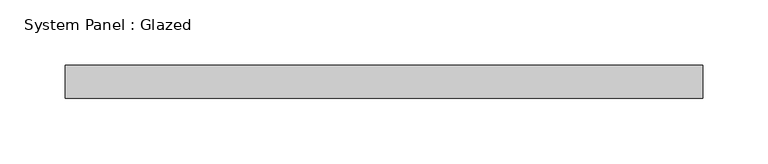
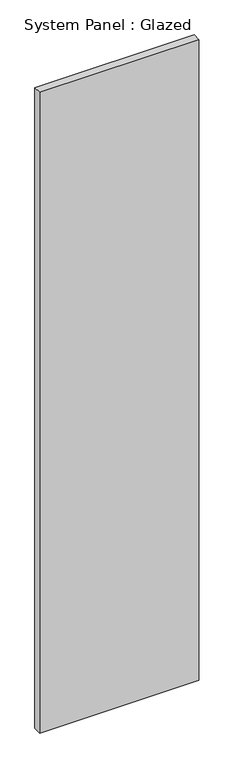
"""IFC4 building model written with IfcOpenShell, lengths in millimetres: plate geometry, System Panel : Glazed."""

from ifc_helpers import new_model, si_unit, origin, origin_with_axes, place, context, project, spatial, polyline, outline, extrude, source, transform, mapped, element, save


def system_panel_glazed_b4762422(model_context):
    return source(origin(), model_context, "Body", "SweptSolid", [
        extrude(outline(polyline([(244.9190503, -44.45), (-244.9190503, -44.45), (-244.9190503, -19.05), (244.9190503, -19.05), (244.9190503, -44.45)])), origin_with_axes(), (0.0, 0.0, 1.0), 2082.8),
    ])


if __name__ == "__main__":
    model = new_model("IFC4")
    model_context = context("Model", 3, world=origin())
    ifc_project = project(units=[si_unit("LENGTHUNIT", "METRE", prefix="MILLI")], contexts=[model_context])
    site = spatial("IfcSite", under=ifc_project)
    building = spatial("IfcBuilding", under=site)
    placement = place(None, origin())
    system_panel_glazed_shape = system_panel_glazed_b4762422(model_context)
    element("IfcPlate", 1, ObjectType="System Panel : Glazed", at=placement, inside=building, context=model_context, shape_type="MappedRepresentation", body=[
        mapped(system_panel_glazed_shape, transform((0.0, 0.0, 0.0), x_axis=(1.0, 0.0, 0.0), y_axis=(0.0, 1.0, 0.0), z_axis=(0.0, 0.0, 1.0))),
    ])
    save(model, "model.ifc")

# Revit data of these elements
# Type "System Panel : Glazed"
#   Construction Type Id = "GSP4R"
#   Analytic Construction = "1/8 in Pilkington single glazing"
#   Visual Light Transmittance = 0.9
#   Solar Heat Gain Coefficient = 0.86
#   Heat Transfer Coefficient (U) = 1.18115 BTU/(h·ft²·°F)
#   Define Thermal Properties by = 1
# Element 1 (IfcPlate, "System Panel : Glazed")
#   Materials on its faces: "Glass"
# Materials
#   "Glass": class "Glass", colour RGB 0 128 192, transparency 0.75, Description = "Soda Lime Glass", Cost = 0
